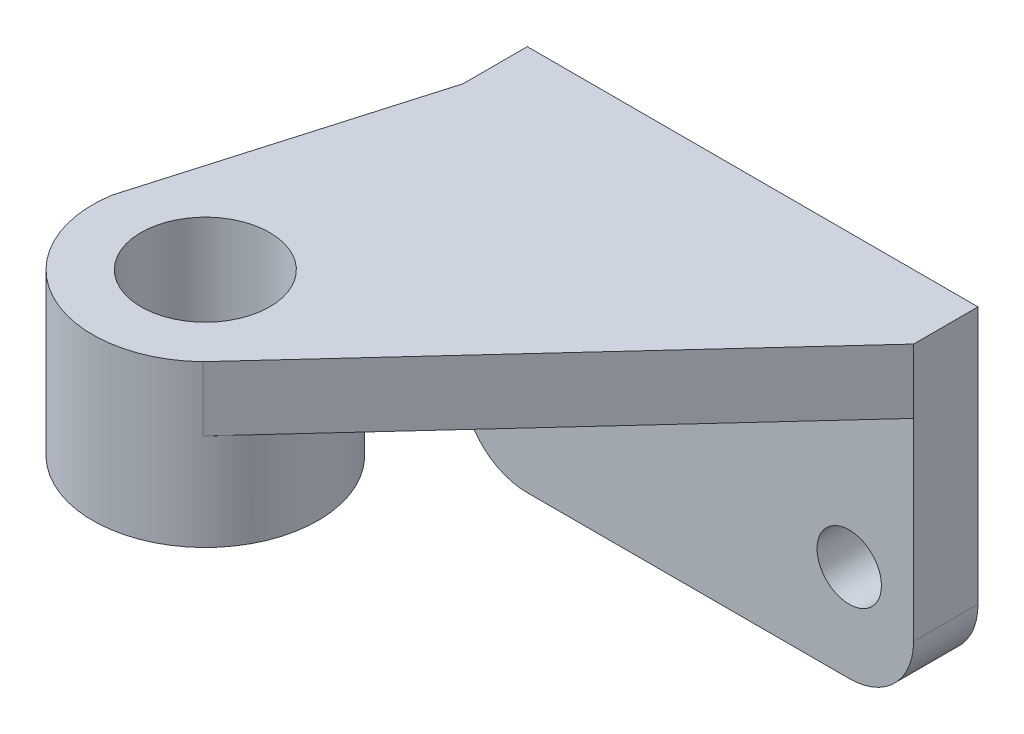
ISO-10303-21;
HEADER;
FILE_DESCRIPTION(('STEP AP214'),'2;1');
FILE_NAME('part.step','',(''),(''),'','','');
FILE_SCHEMA(('AUTOMOTIVE_DESIGN { 1 0 10303 214 1 1 1 1 }'));
ENDSEC;
DATA;
#1=APPLICATION_CONTEXT('core data for automotive mechanical design processes');
#2=APPLICATION_PROTOCOL_DEFINITION('international standard','automotive_design',2000,#1);
#3=PRODUCT_CONTEXT('',#1,'mechanical');
#4=PRODUCT('Part','Part','',(#3));
#5=PRODUCT_RELATED_PRODUCT_CATEGORY('part','',(#4));
#6=PRODUCT_DEFINITION_FORMATION('','',#4);
#7=PRODUCT_DEFINITION_CONTEXT('part definition',#1,'design');
#8=PRODUCT_DEFINITION('design','',#6,#7);
#9=PRODUCT_DEFINITION_SHAPE('','',#8);
#10=(LENGTH_UNIT() NAMED_UNIT(*) SI_UNIT(.MILLI.,.METRE.));
#11=(NAMED_UNIT(*) PLANE_ANGLE_UNIT() SI_UNIT($,.RADIAN.));
#12=(NAMED_UNIT(*) SI_UNIT($,.STERADIAN.) SOLID_ANGLE_UNIT());
#13=UNCERTAINTY_MEASURE_WITH_UNIT(LENGTH_MEASURE(1.E-05),#10,'distance_accuracy_value','');
#14=(GEOMETRIC_REPRESENTATION_CONTEXT(3) GLOBAL_UNCERTAINTY_ASSIGNED_CONTEXT((#13)) GLOBAL_UNIT_ASSIGNED_CONTEXT((#10,
#11,#12)) REPRESENTATION_CONTEXT('',''));
#15=CARTESIAN_POINT('',(0.,0.,0.));
#16=DIRECTION('',(0.,0.,1.));
#17=DIRECTION('',(1.,0.,0.));
#18=AXIS2_PLACEMENT_3D('',#15,#16,#17);
#19=CARTESIAN_POINT('',(0.,-10.,0.));
#20=DIRECTION('',(0.,1.,0.));
#21=DIRECTION('',(0.,0.,1.));
#22=AXIS2_PLACEMENT_3D('',#19,#20,#21);
#23=PLANE('',#22);
#24=CARTESIAN_POINT('',(5.,-10.,55.));
#25=DIRECTION('',(0.,1.,0.));
#26=DIRECTION('',(0.,0.,1.));
#27=AXIS2_PLACEMENT_3D('',#24,#25,#26);
#28=CIRCLE('',#27,17.5);
#29=CARTESIAN_POINT('',(-11.0720481416097,-10.,48.0761810730074));
#30=VERTEX_POINT('',#29);
#31=CARTESIAN_POINT('',(18.5651581010019,-10.,66.0560610388521));
#32=VERTEX_POINT('',#31);
#33=EDGE_CURVE('E11',#30,#32,#28,.F.);
#34=ORIENTED_EDGE('',*,*,#33,.F.);
#35=DIRECTION('',(-0.279221211302421,0.,0.96022680402018));
#36=VECTOR('',#35,1.);
#37=CARTESIAN_POINT('',(2.68115691343567,-10.,0.77964484841191));
#38=LINE('',#37,#36);
#39=CARTESIAN_POINT('',(0.,-10.,10.));
#40=VERTEX_POINT('',#39);
#41=EDGE_CURVE('E182',#40,#30,#38,.T.);
#42=ORIENTED_EDGE('',*,*,#41,.F.);
#43=DIRECTION('',(1.,0.,0.));
#44=VECTOR('',#43,1.);
#45=CARTESIAN_POINT('',(0.,-10.,10.));
#46=LINE('',#45,#44);
#47=CARTESIAN_POINT('',(70.,-10.,10.));
#48=VERTEX_POINT('',#47);
#49=EDGE_CURVE('E65',#40,#48,#46,.T.);
#50=ORIENTED_EDGE('',*,*,#49,.T.);
#51=DIRECTION('',(-0.676082532946038,0.,0.736825901176981));
#52=VECTOR('',#51,1.);
#53=CARTESIAN_POINT('',(42.9854198212487,-10.,39.4417344261059));
#54=LINE('',#53,#52);
#55=EDGE_CURVE('E195',#48,#32,#54,.T.);
#56=ORIENTED_EDGE('',*,*,#55,.T.);
#57=EDGE_LOOP('',(#34,#42,#50,#56));
#58=FACE_BOUND('',#57,.T.);
#59=ADVANCED_FACE('F50',(#58),#23,.F.);
#60=CARTESIAN_POINT('',(0.,0.,10.));
#61=DIRECTION('',(0.,-1.,0.));
#62=DIRECTION('',(0.,0.,-1.));
#63=AXIS2_PLACEMENT_3D('',#60,#61,#62);
#64=PLANE('',#63);
#65=CARTESIAN_POINT('',(5.,0.,55.));
#66=DIRECTION('',(0.,-1.,0.));
#67=DIRECTION('',(0.,0.,-1.));
#68=AXIS2_PLACEMENT_3D('',#65,#66,#67);
#69=CIRCLE('',#68,10.);
#70=CARTESIAN_POINT('',(5.,0.,45.));
#71=VERTEX_POINT('',#70);
#72=EDGE_CURVE('E286',#71,#71,#69,.T.);
#73=ORIENTED_EDGE('',*,*,#72,.T.);
#74=EDGE_LOOP('',(#73));
#75=FACE_BOUND('',#74,.T.);
#76=DIRECTION('',(-1.,0.,0.));
#77=VECTOR('',#76,1.);
#78=CARTESIAN_POINT('',(0.,0.,0.));
#79=LINE('',#78,#77);
#80=CARTESIAN_POINT('',(70.,0.,0.));
#81=VERTEX_POINT('',#80);
#82=CARTESIAN_POINT('',(0.,0.,0.));
#83=VERTEX_POINT('',#82);
#84=EDGE_CURVE('E145',#81,#83,#79,.T.);
#85=ORIENTED_EDGE('',*,*,#84,.T.);
#86=DIRECTION('',(0.,0.,-1.));
#87=VECTOR('',#86,1.);
#88=CARTESIAN_POINT('',(0.,0.,10.));
#89=LINE('',#88,#87);
#90=CARTESIAN_POINT('',(0.,0.,10.));
#91=VERTEX_POINT('',#90);
#92=EDGE_CURVE('E54',#91,#83,#89,.T.);
#93=ORIENTED_EDGE('',*,*,#92,.F.);
#94=DIRECTION('',(-0.279221211302421,0.,0.96022680402018));
#95=VECTOR('',#94,1.);
#96=CARTESIAN_POINT('',(2.68115691343567,0.,0.77964484841191));
#97=LINE('',#96,#95);
#98=CARTESIAN_POINT('',(-12.2787192308994,0.,52.2258583778498));
#99=VERTEX_POINT('',#98);
#100=EDGE_CURVE('E181',#91,#99,#97,.T.);
#101=ORIENTED_EDGE('',*,*,#100,.T.);
#102=CARTESIAN_POINT('',(5.,0.,55.));
#103=DIRECTION('',(0.,1.,0.));
#104=DIRECTION('',(0.,0.,1.));
#105=AXIS2_PLACEMENT_3D('',#102,#103,#104);
#106=CIRCLE('',#105,17.5);
#107=CARTESIAN_POINT('',(17.179494078165,0.,67.5662215482596));
#108=VERTEX_POINT('',#107);
#109=EDGE_CURVE('E205',#99,#108,#106,.T.);
#110=ORIENTED_EDGE('',*,*,#109,.T.);
#111=DIRECTION('',(-0.676082532946038,0.,0.736825901176981));
#112=VECTOR('',#111,1.);
#113=CARTESIAN_POINT('',(42.9854198212487,0.,39.4417344261059));
#114=LINE('',#113,#112);
#115=CARTESIAN_POINT('',(70.,0.,10.));
#116=VERTEX_POINT('',#115);
#117=EDGE_CURVE('E193',#116,#108,#114,.T.);
#118=ORIENTED_EDGE('',*,*,#117,.F.);
#119=DIRECTION('',(0.,0.,-1.));
#120=VECTOR('',#119,1.);
#121=CARTESIAN_POINT('',(70.,0.,10.));
#122=LINE('',#121,#120);
#123=EDGE_CURVE('E72',#116,#81,#122,.T.);
#124=ORIENTED_EDGE('',*,*,#123,.T.);
#125=EDGE_LOOP('',(#85,#93,#101,#110,#118,#124));
#126=FACE_BOUND('',#125,.T.);
#127=ADVANCED_FACE('F47',(#75,#126),#64,.F.);
#128=CARTESIAN_POINT('',(0.,0.,10.));
#129=DIRECTION('',(1.,0.,0.));
#130=DIRECTION('',(0.,0.,-1.));
#131=AXIS2_PLACEMENT_3D('',#128,#129,#130);
#132=PLANE('',#131);
#133=DIRECTION('',(0.,-1.,0.));
#134=VECTOR('',#133,1.);
#135=CARTESIAN_POINT('',(0.,0.,0.));
#136=LINE('',#135,#134);
#137=CARTESIAN_POINT('',(0.,-40.,0.));
#138=VERTEX_POINT('',#137);
#139=EDGE_CURVE('E150',#83,#138,#136,.T.);
#140=ORIENTED_EDGE('',*,*,#139,.T.);
#141=DIRECTION('',(0.,0.,-1.));
#142=VECTOR('',#141,1.);
#143=CARTESIAN_POINT('',(0.,-40.,10.));
#144=LINE('',#143,#142);
#145=CARTESIAN_POINT('',(0.,-40.,10.));
#146=VERTEX_POINT('',#145);
#147=EDGE_CURVE('E159',#146,#138,#144,.T.);
#148=ORIENTED_EDGE('',*,*,#147,.F.);
#149=DIRECTION('',(0.,-1.,0.));
#150=VECTOR('',#149,1.);
#151=CARTESIAN_POINT('',(0.,0.,10.));
#152=LINE('',#151,#150);
#153=EDGE_CURVE('E156',#40,#146,#152,.T.);
#154=ORIENTED_EDGE('',*,*,#153,.F.);
#155=EDGE_CURVE('E102',#91,#40,#152,.T.);
#156=ORIENTED_EDGE('',*,*,#155,.F.);
#157=ORIENTED_EDGE('',*,*,#92,.T.);
#158=EDGE_LOOP('',(#140,#148,#154,#156,#157));
#159=FACE_BOUND('',#158,.T.);
#160=ADVANCED_FACE('F165',(#159),#132,.F.);
#161=CARTESIAN_POINT('',(10.,-40.,10.));
#162=DIRECTION('',(0.,0.,-1.));
#163=DIRECTION('',(-1.,0.,0.));
#164=AXIS2_PLACEMENT_3D('',#161,#162,#163);
#165=CYLINDRICAL_SURFACE('',#164,10.);
#166=CARTESIAN_POINT('',(10.,-40.,0.));
#167=DIRECTION('',(0.,0.,1.));
#168=DIRECTION('',(1.,0.,0.));
#169=AXIS2_PLACEMENT_3D('',#166,#167,#168);
#170=CIRCLE('',#169,10.);
#171=CARTESIAN_POINT('',(10.,-50.,0.));
#172=VERTEX_POINT('',#171);
#173=EDGE_CURVE('E147',#138,#172,#170,.T.);
#174=ORIENTED_EDGE('',*,*,#173,.T.);
#175=DIRECTION('',(0.,0.,-1.));
#176=VECTOR('',#175,1.);
#177=CARTESIAN_POINT('',(10.,-50.,10.));
#178=LINE('',#177,#176);
#179=CARTESIAN_POINT('',(10.,-50.,10.));
#180=VERTEX_POINT('',#179);
#181=EDGE_CURVE('E134',#180,#172,#178,.T.);
#182=ORIENTED_EDGE('',*,*,#181,.F.);
#183=CARTESIAN_POINT('',(10.,-40.,10.));
#184=DIRECTION('',(0.,0.,1.));
#185=DIRECTION('',(1.,0.,0.));
#186=AXIS2_PLACEMENT_3D('',#183,#184,#185);
#187=CIRCLE('',#186,10.);
#188=EDGE_CURVE('E125',#146,#180,#187,.T.);
#189=ORIENTED_EDGE('',*,*,#188,.F.);
#190=ORIENTED_EDGE('',*,*,#147,.T.);
#191=EDGE_LOOP('',(#174,#182,#189,#190));
#192=FACE_BOUND('',#191,.T.);
#193=ADVANCED_FACE('F173',(#192),#165,.T.);
#194=CARTESIAN_POINT('',(10.,-50.,10.));
#195=DIRECTION('',(0.,1.,0.));
#196=DIRECTION('',(0.,0.,1.));
#197=AXIS2_PLACEMENT_3D('',#194,#195,#196);
#198=PLANE('',#197);
#199=DIRECTION('',(1.,0.,0.));
#200=VECTOR('',#199,1.);
#201=CARTESIAN_POINT('',(10.,-50.,0.));
#202=LINE('',#201,#200);
#203=CARTESIAN_POINT('',(60.,-50.,0.));
#204=VERTEX_POINT('',#203);
#205=EDGE_CURVE('E132',#172,#204,#202,.T.);
#206=ORIENTED_EDGE('',*,*,#205,.T.);
#207=DIRECTION('',(0.,0.,-1.));
#208=VECTOR('',#207,1.);
#209=CARTESIAN_POINT('',(60.,-50.,10.));
#210=LINE('',#209,#208);
#211=CARTESIAN_POINT('',(60.,-50.,10.));
#212=VERTEX_POINT('',#211);
#213=EDGE_CURVE('E126',#212,#204,#210,.T.);
#214=ORIENTED_EDGE('',*,*,#213,.F.);
#215=DIRECTION('',(1.,0.,0.));
#216=VECTOR('',#215,1.);
#217=CARTESIAN_POINT('',(10.,-50.,10.));
#218=LINE('',#217,#216);
#219=EDGE_CURVE('E113',#180,#212,#218,.T.);
#220=ORIENTED_EDGE('',*,*,#219,.F.);
#221=ORIENTED_EDGE('',*,*,#181,.T.);
#222=EDGE_LOOP('',(#206,#214,#220,#221));
#223=FACE_BOUND('',#222,.T.);
#224=ADVANCED_FACE('F129',(#223),#198,.F.);
#225=CARTESIAN_POINT('',(60.,-40.,10.));
#226=DIRECTION('',(0.,0.,-1.));
#227=DIRECTION('',(-1.,0.,0.));
#228=AXIS2_PLACEMENT_3D('',#225,#226,#227);
#229=CYLINDRICAL_SURFACE('',#228,10.);
#230=CARTESIAN_POINT('',(60.,-40.,0.));
#231=DIRECTION('',(0.,0.,1.));
#232=DIRECTION('',(1.,0.,0.));
#233=AXIS2_PLACEMENT_3D('',#230,#231,#232);
#234=CIRCLE('',#233,10.);
#235=CARTESIAN_POINT('',(70.,-40.,0.));
#236=VERTEX_POINT('',#235);
#237=EDGE_CURVE('E153',#204,#236,#234,.T.);
#238=ORIENTED_EDGE('',*,*,#237,.T.);
#239=DIRECTION('',(0.,0.,-1.));
#240=VECTOR('',#239,1.);
#241=CARTESIAN_POINT('',(70.,-40.,10.));
#242=LINE('',#241,#240);
#243=CARTESIAN_POINT('',(70.,-40.,10.));
#244=VERTEX_POINT('',#243);
#245=EDGE_CURVE('E131',#244,#236,#242,.T.);
#246=ORIENTED_EDGE('',*,*,#245,.F.);
#247=CARTESIAN_POINT('',(60.,-40.,10.));
#248=DIRECTION('',(0.,0.,1.));
#249=DIRECTION('',(1.,0.,0.));
#250=AXIS2_PLACEMENT_3D('',#247,#248,#249);
#251=CIRCLE('',#250,10.);
#252=EDGE_CURVE('E119',#212,#244,#251,.T.);
#253=ORIENTED_EDGE('',*,*,#252,.F.);
#254=ORIENTED_EDGE('',*,*,#213,.T.);
#255=EDGE_LOOP('',(#238,#246,#253,#254));
#256=FACE_BOUND('',#255,.T.);
#257=ADVANCED_FACE('F140',(#256),#229,.T.);
#258=CARTESIAN_POINT('',(70.,0.,10.));
#259=DIRECTION('',(-1.,0.,0.));
#260=DIRECTION('',(0.,0.,1.));
#261=AXIS2_PLACEMENT_3D('',#258,#259,#260);
#262=PLANE('',#261);
#263=DIRECTION('',(0.,1.,0.));
#264=VECTOR('',#263,1.);
#265=CARTESIAN_POINT('',(70.,0.,0.));
#266=LINE('',#265,#264);
#267=EDGE_CURVE('E100',#236,#81,#266,.T.);
#268=ORIENTED_EDGE('',*,*,#267,.T.);
#269=ORIENTED_EDGE('',*,*,#123,.F.);
#270=DIRECTION('',(0.,1.,0.));
#271=VECTOR('',#270,1.);
#272=CARTESIAN_POINT('',(70.,-10.,10.));
#273=LINE('',#272,#271);
#274=EDGE_CURVE('E146',#48,#116,#273,.T.);
#275=ORIENTED_EDGE('',*,*,#274,.F.);
#276=DIRECTION('',(0.,1.,0.));
#277=VECTOR('',#276,1.);
#278=CARTESIAN_POINT('',(70.,0.,10.));
#279=LINE('',#278,#277);
#280=EDGE_CURVE('E138',#244,#48,#279,.T.);
#281=ORIENTED_EDGE('',*,*,#280,.F.);
#282=ORIENTED_EDGE('',*,*,#245,.T.);
#283=EDGE_LOOP('',(#268,#269,#275,#281,#282));
#284=FACE_BOUND('',#283,.T.);
#285=ADVANCED_FACE('F236',(#284),#262,.F.);
#286=CARTESIAN_POINT('',(60.,-40.,10.));
#287=DIRECTION('',(0.,0.,1.));
#288=DIRECTION('',(1.,0.,0.));
#289=AXIS2_PLACEMENT_3D('',#286,#287,#288);
#290=PLANE('',#289);
#291=CARTESIAN_POINT('',(10.,-35.,10.));
#292=DIRECTION('',(0.,0.,1.));
#293=DIRECTION('',(1.,0.,0.));
#294=AXIS2_PLACEMENT_3D('',#291,#292,#293);
#295=CIRCLE('',#294,5.);
#296=CARTESIAN_POINT('',(15.,-35.,10.));
#297=VERTEX_POINT('',#296);
#298=EDGE_CURVE('E280',#297,#297,#295,.T.);
#299=ORIENTED_EDGE('',*,*,#298,.F.);
#300=EDGE_LOOP('',(#299));
#301=FACE_BOUND('',#300,.T.);
#302=CARTESIAN_POINT('',(60.,-35.,10.));
#303=DIRECTION('',(0.,0.,1.));
#304=DIRECTION('',(1.,0.,0.));
#305=AXIS2_PLACEMENT_3D('',#302,#303,#304);
#306=CIRCLE('',#305,5.00000000000001);
#307=CARTESIAN_POINT('',(65.,-35.,10.));
#308=VERTEX_POINT('',#307);
#309=EDGE_CURVE('E279',#308,#308,#306,.T.);
#310=ORIENTED_EDGE('',*,*,#309,.F.);
#311=EDGE_LOOP('',(#310));
#312=FACE_BOUND('',#311,.T.);
#313=ORIENTED_EDGE('',*,*,#49,.F.);
#314=ORIENTED_EDGE('',*,*,#153,.T.);
#315=ORIENTED_EDGE('',*,*,#188,.T.);
#316=ORIENTED_EDGE('',*,*,#219,.T.);
#317=ORIENTED_EDGE('',*,*,#252,.T.);
#318=ORIENTED_EDGE('',*,*,#280,.T.);
#319=EDGE_LOOP('',(#313,#314,#315,#316,#317,#318));
#320=FACE_BOUND('',#319,.T.);
#321=ADVANCED_FACE('F120',(#301,#312,#320),#290,.T.);
#322=CARTESIAN_POINT('',(60.,-40.,0.));
#323=DIRECTION('',(0.,0.,1.));
#324=DIRECTION('',(1.,0.,0.));
#325=AXIS2_PLACEMENT_3D('',#322,#323,#324);
#326=PLANE('',#325);
#327=CARTESIAN_POINT('',(10.,-35.,0.));
#328=DIRECTION('',(0.,0.,1.));
#329=DIRECTION('',(1.,0.,0.));
#330=AXIS2_PLACEMENT_3D('',#327,#328,#329);
#331=CIRCLE('',#330,5.);
#332=CARTESIAN_POINT('',(15.,-35.,0.));
#333=VERTEX_POINT('',#332);
#334=EDGE_CURVE('E275',#333,#333,#331,.T.);
#335=ORIENTED_EDGE('',*,*,#334,.T.);
#336=EDGE_LOOP('',(#335));
#337=FACE_BOUND('',#336,.T.);
#338=CARTESIAN_POINT('',(60.,-35.,0.));
#339=DIRECTION('',(0.,0.,1.));
#340=DIRECTION('',(1.,0.,0.));
#341=AXIS2_PLACEMENT_3D('',#338,#339,#340);
#342=CIRCLE('',#341,5.00000000000001);
#343=CARTESIAN_POINT('',(65.,-35.,0.));
#344=VERTEX_POINT('',#343);
#345=EDGE_CURVE('E274',#344,#344,#342,.T.);
#346=ORIENTED_EDGE('',*,*,#345,.T.);
#347=EDGE_LOOP('',(#346));
#348=FACE_BOUND('',#347,.T.);
#349=ORIENTED_EDGE('',*,*,#84,.F.);
#350=ORIENTED_EDGE('',*,*,#267,.F.);
#351=ORIENTED_EDGE('',*,*,#237,.F.);
#352=ORIENTED_EDGE('',*,*,#205,.F.);
#353=ORIENTED_EDGE('',*,*,#173,.F.);
#354=ORIENTED_EDGE('',*,*,#139,.F.);
#355=EDGE_LOOP('',(#349,#350,#351,#352,#353,#354));
#356=FACE_BOUND('',#355,.T.);
#357=ADVANCED_FACE('F168',(#337,#348,#356),#326,.F.);
#358=CARTESIAN_POINT('',(2.68115691343567,-10.,0.77964484841191));
#359=DIRECTION('',(-0.96022680402018,0.,-0.279221211302421));
#360=DIRECTION('',(-0.279221211302421,0.,0.96022680402018));
#361=AXIS2_PLACEMENT_3D('',#358,#359,#360);
#362=PLANE('',#361);
#363=ORIENTED_EDGE('',*,*,#100,.F.);
#364=ORIENTED_EDGE('',*,*,#155,.T.);
#365=ORIENTED_EDGE('',*,*,#41,.T.);
#366=CARTESIAN_POINT('',(-12.2787192308994,-10.,52.2258583778497));
#367=VERTEX_POINT('',#366);
#368=EDGE_CURVE('E189',#30,#367,#38,.T.);
#369=ORIENTED_EDGE('',*,*,#368,.T.);
#370=DIRECTION('',(0.,1.,0.));
#371=VECTOR('',#370,1.);
#372=CARTESIAN_POINT('',(-12.2787192308994,-10.,52.2258583778498));
#373=LINE('',#372,#371);
#374=EDGE_CURVE('E199',#367,#99,#373,.T.);
#375=ORIENTED_EDGE('',*,*,#374,.T.);
#376=EDGE_LOOP('',(#363,#364,#365,#369,#375));
#377=FACE_BOUND('',#376,.T.);
#378=ADVANCED_FACE('F177',(#377),#362,.T.);
#379=CARTESIAN_POINT('',(42.9854198212487,-10.,39.4417344261059));
#380=DIRECTION('',(-0.736825901176981,0.,-0.676082532946038));
#381=DIRECTION('',(-0.676082532946038,0.,0.736825901176981));
#382=AXIS2_PLACEMENT_3D('',#379,#380,#381);
#383=PLANE('',#382);
#384=ORIENTED_EDGE('',*,*,#117,.T.);
#385=DIRECTION('',(0.,1.,0.));
#386=VECTOR('',#385,1.);
#387=CARTESIAN_POINT('',(17.179494078165,-10.,67.5662215482596));
#388=LINE('',#387,#386);
#389=CARTESIAN_POINT('',(17.179494078165,-10.,67.5662215482596));
#390=VERTEX_POINT('',#389);
#391=EDGE_CURVE('E207',#390,#108,#388,.T.);
#392=ORIENTED_EDGE('',*,*,#391,.F.);
#393=EDGE_CURVE('E188',#32,#390,#54,.T.);
#394=ORIENTED_EDGE('',*,*,#393,.F.);
#395=ORIENTED_EDGE('',*,*,#55,.F.);
#396=ORIENTED_EDGE('',*,*,#274,.T.);
#397=EDGE_LOOP('',(#384,#392,#394,#395,#396));
#398=FACE_BOUND('',#397,.T.);
#399=ADVANCED_FACE('F240',(#398),#383,.F.);
#400=CARTESIAN_POINT('',(5.,-10.,55.));
#401=DIRECTION('',(0.,1.,0.));
#402=DIRECTION('',(0.,0.,1.));
#403=AXIS2_PLACEMENT_3D('',#400,#401,#402);
#404=CYLINDRICAL_SURFACE('',#403,17.5);
#405=ORIENTED_EDGE('',*,*,#109,.F.);
#406=ORIENTED_EDGE('',*,*,#374,.F.);
#407=CARTESIAN_POINT('',(5.,-10.,55.));
#408=DIRECTION('',(0.,-1.,0.));
#409=DIRECTION('',(0.,0.,-1.));
#410=AXIS2_PLACEMENT_3D('',#407,#408,#409);
#411=CIRCLE('',#410,17.5);
#412=EDGE_CURVE('E235',#367,#30,#411,.T.);
#413=ORIENTED_EDGE('',*,*,#412,.T.);
#414=ORIENTED_EDGE('',*,*,#33,.T.);
#415=EDGE_CURVE('E198',#32,#390,#411,.T.);
#416=ORIENTED_EDGE('',*,*,#415,.T.);
#417=ORIENTED_EDGE('',*,*,#391,.T.);
#418=EDGE_LOOP('',(#405,#406,#413,#414,#416,#417));
#419=FACE_BOUND('',#418,.T.);
#420=CARTESIAN_POINT('',(5.,-25.,55.));
#421=DIRECTION('',(0.,-1.,0.));
#422=DIRECTION('',(0.,0.,-1.));
#423=AXIS2_PLACEMENT_3D('',#420,#421,#422);
#424=CIRCLE('',#423,17.5);
#425=CARTESIAN_POINT('',(5.,-25.,37.5));
#426=VERTEX_POINT('',#425);
#427=EDGE_CURVE('E201',#426,#426,#424,.T.);
#428=ORIENTED_EDGE('',*,*,#427,.F.);
#429=EDGE_LOOP('',(#428));
#430=FACE_BOUND('',#429,.T.);
#431=ADVANCED_FACE('F218',(#419,#430),#404,.T.);
#432=CARTESIAN_POINT('',(5.,-10.,55.));
#433=DIRECTION('',(0.,-1.,0.));
#434=DIRECTION('',(0.,0.,-1.));
#435=AXIS2_PLACEMENT_3D('',#432,#433,#434);
#436=PLANE('',#435);
#437=ORIENTED_EDGE('',*,*,#415,.F.);
#438=ORIENTED_EDGE('',*,*,#393,.T.);
#439=EDGE_LOOP('',(#437,#438));
#440=FACE_BOUND('',#439,.T.);
#441=ADVANCED_FACE('F234',(#440),#436,.F.);
#442=CARTESIAN_POINT('',(5.,-25.,55.));
#443=DIRECTION('',(0.,-1.,0.));
#444=DIRECTION('',(0.,0.,-1.));
#445=AXIS2_PLACEMENT_3D('',#442,#443,#444);
#446=PLANE('',#445);
#447=CARTESIAN_POINT('',(5.,-25.,55.));
#448=DIRECTION('',(0.,-1.,0.));
#449=DIRECTION('',(0.,0.,-1.));
#450=AXIS2_PLACEMENT_3D('',#447,#448,#449);
#451=CIRCLE('',#450,10.);
#452=CARTESIAN_POINT('',(5.,-25.,45.));
#453=VERTEX_POINT('',#452);
#454=EDGE_CURVE('E288',#453,#453,#451,.T.);
#455=ORIENTED_EDGE('',*,*,#454,.F.);
#456=EDGE_LOOP('',(#455));
#457=FACE_BOUND('',#456,.T.);
#458=ORIENTED_EDGE('',*,*,#427,.T.);
#459=EDGE_LOOP('',(#458));
#460=FACE_BOUND('',#459,.T.);
#461=ADVANCED_FACE('F294',(#457,#460),#446,.T.);
#462=ORIENTED_EDGE('',*,*,#368,.F.);
#463=ORIENTED_EDGE('',*,*,#412,.F.);
#464=EDGE_LOOP('',(#462,#463));
#465=FACE_BOUND('',#464,.T.);
#466=ADVANCED_FACE('F256',(#465),#436,.F.);
#467=CARTESIAN_POINT('',(5.,0.,55.));
#468=DIRECTION('',(0.,-1.,0.));
#469=DIRECTION('',(0.,0.,-1.));
#470=AXIS2_PLACEMENT_3D('',#467,#468,#469);
#471=CYLINDRICAL_SURFACE('',#470,10.);
#472=ORIENTED_EDGE('',*,*,#72,.F.);
#473=EDGE_LOOP('',(#472));
#474=FACE_BOUND('',#473,.T.);
#475=ORIENTED_EDGE('',*,*,#454,.T.);
#476=EDGE_LOOP('',(#475));
#477=FACE_BOUND('',#476,.T.);
#478=ADVANCED_FACE('F301',(#474,#477),#471,.F.);
#479=CARTESIAN_POINT('',(60.,-35.,0.));
#480=DIRECTION('',(0.,0.,1.));
#481=DIRECTION('',(1.,0.,0.));
#482=AXIS2_PLACEMENT_3D('',#479,#480,#481);
#483=CYLINDRICAL_SURFACE('',#482,5.00000000000001);
#484=ORIENTED_EDGE('',*,*,#345,.F.);
#485=EDGE_LOOP('',(#484));
#486=FACE_BOUND('',#485,.T.);
#487=ORIENTED_EDGE('',*,*,#309,.T.);
#488=EDGE_LOOP('',(#487));
#489=FACE_BOUND('',#488,.T.);
#490=ADVANCED_FACE('F307',(#486,#489),#483,.F.);
#491=CARTESIAN_POINT('',(10.,-35.,0.));
#492=DIRECTION('',(0.,0.,1.));
#493=DIRECTION('',(1.,0.,0.));
#494=AXIS2_PLACEMENT_3D('',#491,#492,#493);
#495=CYLINDRICAL_SURFACE('',#494,5.);
#496=ORIENTED_EDGE('',*,*,#334,.F.);
#497=EDGE_LOOP('',(#496));
#498=FACE_BOUND('',#497,.T.);
#499=ORIENTED_EDGE('',*,*,#298,.T.);
#500=EDGE_LOOP('',(#499));
#501=FACE_BOUND('',#500,.T.);
#502=ADVANCED_FACE('F313',(#498,#501),#495,.F.);
#503=CLOSED_SHELL('',(#59,#127,#160,#193,#224,#257,#285,#321,#357,#378,#399,#431,#441,#461,#466,
#478,#490,#502));
#504=MANIFOLD_SOLID_BREP('B2',#503);
#505=ADVANCED_BREP_SHAPE_REPRESENTATION('',(#18,#504),#14);
#506=SHAPE_DEFINITION_REPRESENTATION(#9,#505);
ENDSEC;
END-ISO-10303-21;
